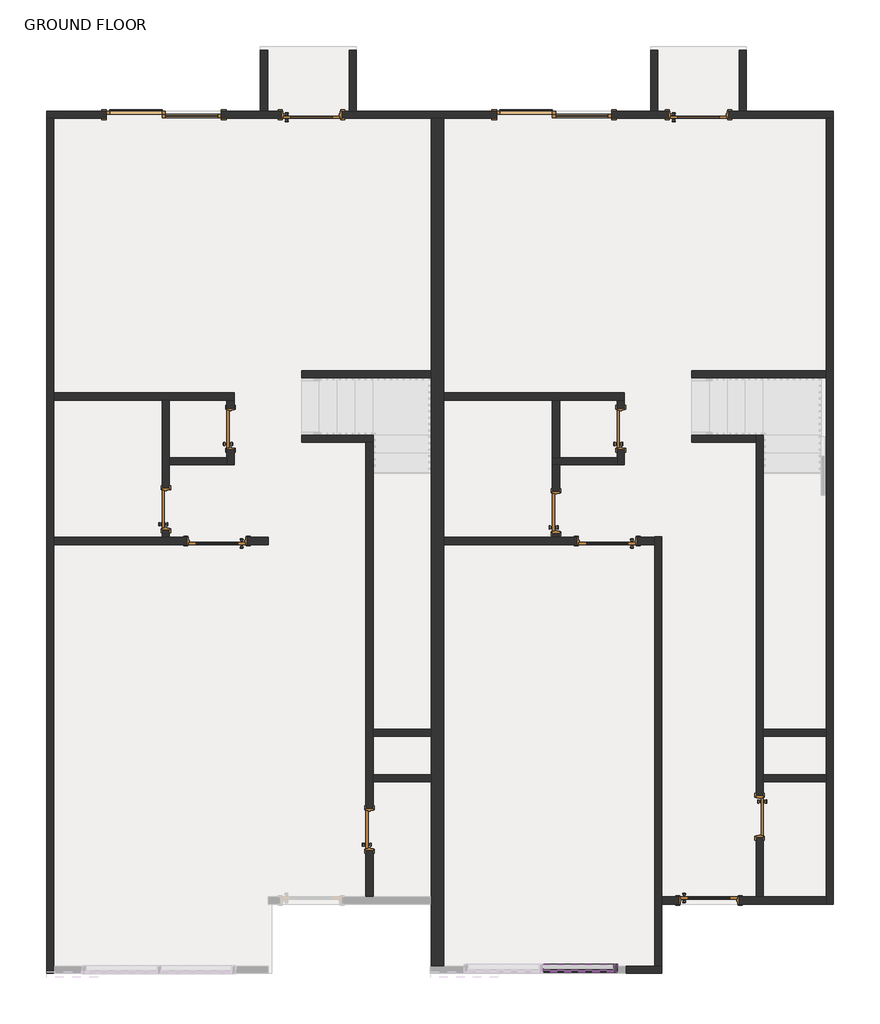
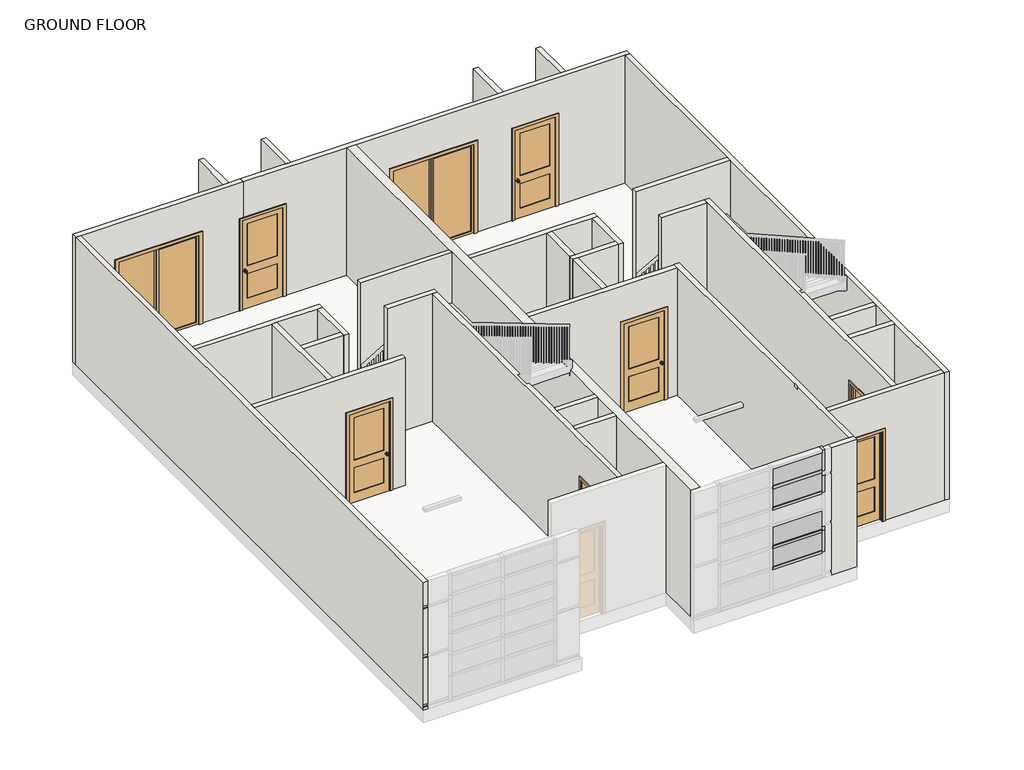
# One storey, part 2 of 4: 33 walls, 13 doors, 8 members, 4 plates.
"""IFC4 building model written with IfcOpenShell, lengths in millimetres."""

from ifc_helpers import new_model, si_unit, frame, origin, place, context, project, spatial, polyline, outline, extrude, faceted_brep, transform, mapped, element, save
from components import door_166d4031, door_049a69ed, door_d4071c8b, door_c25f678d, member_866a01fa, member_7cfea1b5, member_7fd687a9, member_fb13da3b, system_panel_glazed_162183a4, system_panel_glazed_09ecb9ef, system_panel_glazed_28d744da, system_panel_glazed_d671f7fc

model = new_model("IFC4")

# Units and contexts
model_context = context("Model", 3, world=origin())
ifc_project = project(units=[si_unit("LENGTHUNIT", "METRE", prefix="MILLI")], contexts=[model_context])

# Site, building, storey
site = spatial("IfcSite", under=ifc_project)
building = spatial("IfcBuilding", under=site)
storey = spatial("IfcBuildingStorey", under=building, Name="GROUND FLOOR", Elevation=304.8)

# Doors
placement = place(None, origin())
door_shape = door_166d4031(model_context)
element("IfcDoor", 1, ObjectType="Door-Double-Sliding : 72\" x 84\"", at=placement, inside=storey, context=model_context, shape_type="MappedRepresentation", body=[
    mapped(door_shape, transform((-16396.3007021, 8102.2409199, 304.8), x_axis=(1.0, 0.0, 0.0), y_axis=(0.0, 1.0, 0.0), z_axis=(0.0, 0.0, 1.0))),
])
element("IfcDoor", 2, ObjectType="Door-Double-Sliding : 72\" x 84\"", at=placement, inside=storey, context=model_context, shape_type="MappedRepresentation", body=[
    mapped(door_shape, transform((-10187.8860997, 8102.2409199, 304.8), x_axis=(1.0, 0.0, 0.0), y_axis=(0.0, 1.0, 0.0), z_axis=(0.0, 0.0, 1.0))),
])
door_2_shape = door_049a69ed(model_context)
element("IfcDoor", 3, ObjectType="Door-Interior-Single-2_Panel-Wood : 36\" x 84\"", at=placement, inside=storey, context=model_context, shape_type="MappedRepresentation", body=[
    mapped(door_2_shape, transform((-14046.8007021, 8226.0659199, 304.8), x_axis=(1.0, 0.0, 0.0), y_axis=(0.0, 1.0, 0.0), z_axis=(0.0, 0.0, 1.0))),
])
element("IfcDoor", 4, ObjectType="Door-Interior-Single-2_Panel-Wood : 36\" x 84\"", at=placement, inside=storey, context=model_context, shape_type="MappedRepresentation", body=[
    mapped(door_2_shape, transform((-7889.1860997, 8226.0659199, 304.8), x_axis=(1.0, 0.0, 0.0), y_axis=(0.0, 1.0, 0.0), z_axis=(0.0, 0.0, 1.0))),
])
door_3_shape = door_d4071c8b(model_context)
element("IfcDoor", 5, ObjectType="Door-Interior-Single-2_Panel-Wood : 36\" x 84\"", at=placement, inside=storey, context=model_context, shape_type="MappedRepresentation", body=[
    mapped(door_3_shape, transform((-15551.7507021, 1444.2659199, 304.8), x_axis=(-1.0, 0.0, 0.0), y_axis=(0.0, -1.0, 0.0), z_axis=(0.0, 0.0, 1.0))),
])
element("IfcDoor", 6, ObjectType="Door-Interior-Single-2_Panel-Wood : 36\" x 84\"", at=placement, inside=storey, context=model_context, shape_type="MappedRepresentation", body=[
    mapped(door_3_shape, transform((-9343.3360997, 1444.2659199, 304.8), x_axis=(-1.0, 0.0, 0.0), y_axis=(0.0, -1.0, 0.0), z_axis=(0.0, 0.0, 1.0))),
])
element("IfcDoor", 7, ObjectType="Door-Interior-Single-2_Panel-Wood : 36\" x 84\"", at=placement, inside=storey, context=model_context, shape_type="MappedRepresentation", body=[
    mapped(door_3_shape, transform((-7724.0860997, -4269.4090831, 304.8), x_axis=(1.0, 0.0, 0.0), y_axis=(0.0, 1.0, 0.0), z_axis=(0.0, 0.0, 1.0))),
])
door_4_shape = door_c25f678d(model_context)
element("IfcDoor", 8, ObjectType="Door-Interior-Single-Flush_Panel-Wood : 24\" x 84\"", at=placement, inside=storey, context=model_context, shape_type="MappedRepresentation", body=[
    mapped(door_4_shape, transform((-16367.7257021, 1955.4409199, 304.8), x_axis=(0.0, 1.0, 0.0), y_axis=(-1.0, 0.0, 0.0), z_axis=(0.0, 0.0, 1.0))),
])
element("IfcDoor", 9, ObjectType="Door-Interior-Single-Flush_Panel-Wood : 24\" x 84\"", at=placement, inside=storey, context=model_context, shape_type="MappedRepresentation", body=[
    mapped(door_4_shape, transform((-15339.0257021, 3231.7909199, 304.8), x_axis=(0.0, 1.0, 0.0), y_axis=(-1.0, 0.0, 0.0), z_axis=(0.0, 0.0, 1.0))),
])
element("IfcDoor", 10, ObjectType="Door-Interior-Single-Flush_Panel-Wood : 24\" x 84\"", at=placement, inside=storey, context=model_context, shape_type="MappedRepresentation", body=[
    mapped(door_4_shape, transform((-10159.3110997, 1904.6409199, 304.8), x_axis=(0.0, 1.0, 0.0), y_axis=(-1.0, 0.0, 0.0), z_axis=(0.0, 0.0, 1.0))),
])
element("IfcDoor", 11, ObjectType="Door-Interior-Single-Flush_Panel-Wood : 24\" x 84\"", at=placement, inside=storey, context=model_context, shape_type="MappedRepresentation", body=[
    mapped(door_4_shape, transform((-9130.6110998, 3231.7909199, 304.8), x_axis=(0.0, 1.0, 0.0), y_axis=(-1.0, 0.0, 0.0), z_axis=(0.0, 0.0, 1.0))),
])
element("IfcDoor", 12, ObjectType="Door-Interior-Single-Flush_Panel-Wood : 24\" x 84\"", at=placement, inside=storey, context=model_context, shape_type="MappedRepresentation", body=[
    mapped(door_4_shape, transform((-13129.2257021, -3142.284083, 304.8), x_axis=(0.0, 1.0, 0.0), y_axis=(-1.0, 0.0, 0.0), z_axis=(0.0, 0.0, 1.0))),
])
element("IfcDoor", 13, ObjectType="Door-Interior-Single-Flush_Panel-Wood : 24\" x 84\"", at=placement, inside=storey, context=model_context, shape_type="MappedRepresentation", body=[
    mapped(door_4_shape, transform((-6914.4610997, -2939.0840831, 304.8), x_axis=(0.0, -1.0, 0.0), y_axis=(1.0, 0.0, 0.0), z_axis=(0.0, 0.0, 1.0))),
])

# Members
member_shape = member_866a01fa(model_context)
element("IfcMember", 14, ObjectType="Rectangular Mullion : 2.5\" x 5\" rectangular", at=placement, inside=storey, context=model_context, shape_type="MappedRepresentation", body=[
    mapped(member_shape, transform((-9240.0344894, -5353.4090801, 2336.8), x_axis=(0.0, 0.0, 1.0), y_axis=(0.0, -1.0, 0.0), z_axis=(1.0, 0.0, 0.0))),
])
element("IfcMember", 15, ObjectType="Rectangular Mullion : 2.5\" x 5\" rectangular", at=placement, inside=storey, context=model_context, shape_type="MappedRepresentation", body=[
    mapped(member_shape, transform((-9240.0344894, -5353.4090801, 914.4), x_axis=(0.0, 0.0, 1.0), y_axis=(0.0, -1.0, 0.0), z_axis=(1.0, 0.0, 0.0))),
])
element("IfcMember", 16, ObjectType="Rectangular Mullion : 2.5\" x 5\" rectangular", at=placement, inside=storey, context=model_context, shape_type="MappedRepresentation", body=[
    mapped(member_shape, transform((-9240.0344894, -5353.4090801, 2844.8), x_axis=(0.0, 0.0, 1.0), y_axis=(0.0, -1.0, 0.0), z_axis=(1.0, 0.0, 0.0))),
])
element("IfcMember", 17, ObjectType="Rectangular Mullion : 2.5\" x 5\" rectangular", at=placement, inside=storey, context=model_context, shape_type="MappedRepresentation", body=[
    mapped(member_shape, transform((-9240.0344894, -5353.4090801, 1422.4), x_axis=(0.0, 0.0, 1.0), y_axis=(0.0, -1.0, 0.0), z_axis=(1.0, 0.0, 0.0))),
])
member_2_shape = member_7cfea1b5(model_context)
element("IfcMember", 18, ObjectType="Rectangular Mullion : 2.5\" x 5\" rectangular", at=placement, inside=storey, context=model_context, shape_type="MappedRepresentation", body=[
    mapped(member_2_shape, transform((-9176.5344894, -5353.4090801, 2336.8), x_axis=(1.0, 0.0, 0.0), y_axis=(0.0, -1.0, 0.0), z_axis=(0.0, 0.0, -1.0))),
])
member_3_shape = member_7fd687a9(model_context)
element("IfcMember", 19, ObjectType="Rectangular Mullion : 2.5\" x 5\" rectangular", at=placement, inside=storey, context=model_context, shape_type="MappedRepresentation", body=[
    mapped(member_3_shape, transform((-9176.5344894, -5353.4090801, 2844.8), x_axis=(1.0, 0.0, 0.0), y_axis=(0.0, -1.0, 0.0), z_axis=(0.0, 0.0, -1.0))),
])
element("IfcMember", 20, ObjectType="Rectangular Mullion : 2.5\" x 5\" rectangular", at=placement, inside=storey, context=model_context, shape_type="MappedRepresentation", body=[
    mapped(member_3_shape, transform((-9176.5344894, -5353.4090801, 914.4), x_axis=(1.0, 0.0, 0.0), y_axis=(0.0, -1.0, 0.0), z_axis=(0.0, 0.0, -1.0))),
])
member_4_shape = member_fb13da3b(model_context)
element("IfcMember", 21, ObjectType="Rectangular Mullion : 2.5\" x 5\" rectangular", at=placement, inside=storey, context=model_context, shape_type="MappedRepresentation", body=[
    mapped(member_4_shape, transform((-9176.5344894, -5353.4090801, 1422.4), x_axis=(1.0, 0.0, 0.0), y_axis=(0.0, -1.0, 0.0), z_axis=(0.0, 0.0, -1.0))),
])

# Plates
system_panel_glazed_shape = system_panel_glazed_162183a4(model_context)
element("IfcPlate", 22, ObjectType="System Panel : Glazed", at=placement, inside=storey, context=model_context, shape_type="MappedRepresentation", body=[
    mapped(system_panel_glazed_shape, transform((-9802.0094894, -5353.4090801, 2368.55), x_axis=(1.0, 0.0, 0.0), y_axis=(0.0, 1.0, 0.0), z_axis=(0.0, 0.0, 1.0))),
])
system_panel_glazed_2_shape = system_panel_glazed_09ecb9ef(model_context)
element("IfcPlate", 23, ObjectType="System Panel : Glazed", at=placement, inside=storey, context=model_context, shape_type="MappedRepresentation", body=[
    mapped(system_panel_glazed_2_shape, transform((-9802.0094894, -5353.4090801, 2876.55), x_axis=(1.0, 0.0, 0.0), y_axis=(0.0, 1.0, 0.0), z_axis=(0.0, 0.0, 1.0))),
])
system_panel_glazed_3_shape = system_panel_glazed_28d744da(model_context)
element("IfcPlate", 24, ObjectType="System Panel : Glazed", at=placement, inside=storey, context=model_context, shape_type="MappedRepresentation", body=[
    mapped(system_panel_glazed_3_shape, transform((-9802.0094894, -5353.4090801, 946.15), x_axis=(1.0, 0.0, 0.0), y_axis=(0.0, 1.0, 0.0), z_axis=(0.0, 0.0, 1.0))),
])
system_panel_glazed_4_shape = system_panel_glazed_d671f7fc(model_context)
element("IfcPlate", 25, ObjectType="System Panel : Glazed", at=placement, inside=storey, context=model_context, shape_type="MappedRepresentation", body=[
    mapped(system_panel_glazed_4_shape, transform((-9802.0094894, -5353.4090801, 1454.15), x_axis=(1.0, 0.0, 0.0), y_axis=(0.0, 1.0, 0.0), z_axis=(0.0, 0.0, 1.0))),
])

# Walls
element("IfcWall", 26, at=placement, inside=storey, context=model_context, shape_type="Brep", body=[
    faceted_brep([(-18263.2007021, 8286.3909199, 3352.8), (-14859.6007021, 8286.3909199, 3352.8), (-14745.3007021, 8286.3909199, 3352.8), (-14478.6007021, 8286.3909199, 3352.8), (-14478.6007021, 8286.3909199, 2463.8), (-14529.4007021, 8286.3909199, 2463.8), (-14529.4007021, 8286.3909199, 304.8), (-14745.3007021, 8286.3909199, 304.8), (-14859.6007021, 8286.3909199, 304.8), (-15481.9007021, 8286.3909199, 304.8), (-15481.9007021, 8286.3909199, 2438.4), (-17310.7007021, 8286.3909199, 2438.4), (-17310.7007021, 8286.3909199, 304.8), (-18263.2007021, 8286.3909199, 304.8), (-14478.6007021, 8172.0909199, 3352.8), (-18148.9007021, 8172.0909199, 3352.8), (-18263.2007021, 8172.0909199, 3352.8), (-18263.2007021, 8172.0909199, 304.8), (-18148.9007021, 8172.0909199, 304.8), (-17310.7007021, 8172.0909199, 304.8), (-17310.7007021, 8172.0909199, 2438.4), (-15481.9007021, 8172.0909199, 2438.4), (-15481.9007021, 8172.0909199, 304.8), (-14529.4007021, 8172.0909199, 304.8), (-14529.4007021, 8172.0909199, 2463.8), (-14478.6007021, 8172.0909199, 2463.8)], [[[0, 1, 2, 3, 4, 5, 6, 7, 8, 9, 10, 11, 12, 13]], [[14, 15, 16, 17, 18, 19, 20, 21, 22, 23, 24, 25]], [[17, 13, 12, 19, 18]], [[22, 9, 8, 7, 6, 23]], [[3, 2, 1, 0, 16, 15, 14]], [[3, 14, 25, 4]], [[0, 13, 17, 16]], [[12, 11, 20, 19]], [[10, 9, 22, 21]], [[11, 10, 21, 20]], [[24, 5, 4, 25]], [[5, 24, 23, 6]]]),
])
element("IfcWall", 27, at=placement, inside=storey, context=model_context, shape_type="Brep", body=[
    faceted_brep([(-18263.2007021, 8172.0909199, 304.8), (-18263.2007021, -5429.6090801, 304.8), (-18263.2007021, -5429.6090801, 368.3), (-18263.2007021, -5404.2090801, 368.3), (-18263.2007021, -5404.2090801, 436.0333333), (-18263.2007021, -5429.6090801, 436.0333333), (-18263.2007021, -5429.6090801, 1544.32), (-18263.2007021, -5404.2090801, 1544.32), (-18263.2007021, -5404.2090801, 1612.0533333), (-18263.2007021, -5429.6090801, 1612.0533333), (-18263.2007021, -5429.6090801, 2720.34), (-18263.2007021, -5404.2090801, 2720.34), (-18263.2007021, -5404.2090801, 2788.0733333), (-18263.2007021, -5429.6090801, 2788.0733333), (-18263.2007021, -5429.6090801, 3352.8), (-18263.2007021, 8172.0909199, 3352.8), (-18148.9007021, -5429.6090801, 304.8), (-18148.9007021, -5315.3090801, 304.8), (-18148.9007021, 1390.2909199, 304.8), (-18148.9007021, 1504.5909199, 304.8), (-18148.9007021, 3688.9909199, 304.8), (-18148.9007021, 3803.2909199, 304.8), (-18148.9007021, 8172.0909199, 304.8), (-18148.9007021, 8172.0909199, 3352.8), (-18148.9007021, 3803.2909199, 3352.8), (-18148.9007021, 3688.9909199, 3352.8), (-18148.9007021, 1504.5909199, 3352.8), (-18148.9007021, 1390.2909199, 3352.8), (-18148.9007021, -5315.3090801, 3352.8), (-18148.9007021, -5429.6090801, 3352.8), (-18148.9007021, -5429.6090801, 2788.0733333), (-18148.9007021, -5404.2090801, 2788.0733333), (-18148.9007021, -5404.2090801, 2720.34), (-18148.9007021, -5429.6090801, 2720.34), (-18148.9007021, -5429.6090801, 1612.0533333), (-18148.9007021, -5404.2090801, 1612.0533333), (-18148.9007021, -5404.2090801, 1544.32), (-18148.9007021, -5429.6090801, 1544.32), (-18148.9007021, -5429.6090801, 436.0333333), (-18148.9007021, -5404.2090801, 436.0333333), (-18148.9007021, -5404.2090801, 368.3), (-18148.9007021, -5429.6090801, 368.3)], [[[0, 1, 2, 3, 4, 5, 6, 7, 8, 9, 10, 11, 12, 13, 14, 15]], [[16, 17, 18, 19, 20, 21, 22, 23, 24, 25, 26, 27, 28, 29, 30, 31, 32, 33, 34, 35, 36, 37, 38, 39, 40, 41]], [[1, 0, 22, 21, 20, 19, 18, 17, 16]], [[15, 14, 29, 28, 27, 26, 25, 24, 23]], [[0, 15, 23, 22]], [[1, 16, 41, 2]], [[29, 14, 13, 30]], [[5, 38, 37, 6]], [[9, 34, 33, 10]], [[39, 4, 3, 40]], [[40, 3, 2, 41]], [[4, 39, 38, 5]], [[35, 8, 7, 36]], [[36, 7, 6, 37]], [[8, 35, 34, 9]], [[31, 12, 11, 32]], [[32, 11, 10, 33]], [[12, 31, 30, 13]]]),
])
element("IfcWall", 28, at=placement, inside=storey, context=model_context, shape_type="Brep", body=[
    faceted_brep([(-14738.9507021, 1390.2909199, 304.8), (-14738.9507021, 1390.2909199, 3352.8), (-18148.9007021, 1390.2909199, 3352.8), (-18148.9007021, 1390.2909199, 304.8), (-16034.3507021, 1390.2909199, 304.8), (-16034.3507021, 1390.2909199, 2463.8), (-15069.1507021, 1390.2909199, 2463.8), (-15069.1507021, 1390.2909199, 304.8), (-14738.9507021, 1504.5909199, 3352.8), (-14738.9507021, 1504.5909199, 304.8), (-15069.1507021, 1504.5909199, 304.8), (-15069.1507021, 1504.5909199, 2463.8), (-16034.3507021, 1504.5909199, 2463.8), (-16034.3507021, 1504.5909199, 304.8), (-16307.4007021, 1504.5909199, 304.8), (-16421.7007021, 1504.5909199, 304.8), (-18148.9007021, 1504.5909199, 304.8), (-18148.9007021, 1504.5909199, 3352.8), (-16421.7007021, 1504.5909199, 3352.8), (-16307.4007021, 1504.5909199, 3352.8)], [[[0, 1, 2, 3, 4, 5, 6, 7]], [[8, 9, 10, 11, 12, 13, 14, 15, 16, 17, 18, 19]], [[9, 0, 7, 10]], [[3, 16, 15, 14, 13, 4]], [[1, 0, 9, 8]], [[2, 1, 8, 19, 18, 17]], [[3, 2, 17, 16]], [[12, 5, 4, 13]], [[5, 12, 11, 6]], [[6, 11, 10, 7]]]),
])
element("IfcWall", 29, at=placement, inside=storey, context=model_context, shape_type="Brep", body=[
    faceted_brep([(-18148.9007021, 3688.9909199, 304.8), (-16421.7007021, 3688.9909199, 304.8), (-16307.4007021, 3688.9909199, 304.8), (-15393.0007021, 3688.9909199, 304.8), (-15278.7007021, 3688.9909199, 304.8), (-15278.7007021, 3688.9909199, 3352.8), (-15393.0007021, 3688.9909199, 3352.8), (-16307.4007021, 3688.9909199, 3352.8), (-16421.7007021, 3688.9909199, 3352.8), (-18148.9007021, 3688.9909199, 3352.8), (-18148.9007021, 3803.2909199, 304.8), (-18148.9007021, 3803.2909199, 3352.8), (-15278.7007021, 3803.2909199, 3352.8), (-15278.7007021, 3803.2909199, 304.8)], [[[0, 1, 2, 3, 4, 5, 6, 7, 8, 9]], [[10, 11, 12, 13]], [[4, 3, 2, 1, 0, 10, 13]], [[9, 8, 7, 6, 5, 12, 11]], [[0, 9, 11, 10]], [[5, 4, 13, 12]]]),
])
element("IfcWall", 30, at=placement, inside=storey, context=model_context, shape_type="Brep", body=[
    faceted_brep([(-15393.0007021, 2660.2909199, 3352.8), (-15393.0007021, 2774.5909199, 3352.8), (-15393.0007021, 3688.9909199, 3352.8), (-15393.0007021, 3688.9909199, 304.8), (-15393.0007021, 3561.9909199, 304.8), (-15393.0007021, 3561.9909199, 2463.8), (-15393.0007021, 2901.5909199, 2463.8), (-15393.0007021, 2901.5909199, 304.8), (-15393.0007021, 2774.5909199, 304.8), (-15393.0007021, 2660.2909199, 304.8), (-15278.7007021, 3688.9909199, 3352.8), (-15278.7007021, 2660.2909199, 3352.8), (-15278.7007021, 2660.2909199, 304.8), (-15278.7007021, 2901.5909199, 304.8), (-15278.7007021, 2901.5909199, 2463.8), (-15278.7007021, 3561.9909199, 2463.8), (-15278.7007021, 3561.9909199, 304.8), (-15278.7007021, 3688.9909199, 304.8)], [[[0, 1, 2, 3, 4, 5, 6, 7, 8, 9]], [[10, 11, 12, 13, 14, 15, 16, 17]], [[3, 17, 16, 4]], [[12, 9, 8, 7, 13]], [[2, 1, 0, 11, 10]], [[3, 2, 10, 17]], [[0, 9, 12, 11]], [[15, 5, 4, 16]], [[5, 15, 14, 6]], [[6, 14, 13, 7]]]),
])
element("IfcWall", 31, at=placement, inside=storey, context=model_context, shape_type="SweptSolid", body=[
    extrude(outline(polyline([(-16307.4007021, 2774.5909199), (-15393.0007021, 2774.5909199), (-15393.0007021, 2660.2909199), (-16307.4007021, 2660.2909199), (-16307.4007021, 2774.5909199)])), frame((0.0, 0.0, 304.8), z_axis=(0.0, 0.0, 1.0), x_axis=(1.0, 0.0, 0.0)), (0.0, 0.0, 1.0), 3048.0),
])
element("IfcWall", 32, at=placement, inside=storey, context=model_context, shape_type="Brep", body=[
    faceted_brep([(-16421.7007021, 1504.5909199, 3352.8), (-16421.7007021, 3688.9909199, 3352.8), (-16421.7007021, 3688.9909199, 304.8), (-16421.7007021, 2285.6409199, 304.8), (-16421.7007021, 2285.6409199, 2463.8), (-16421.7007021, 1625.2409199, 2463.8), (-16421.7007021, 1625.2409199, 304.8), (-16421.7007021, 1504.5909199, 304.8), (-16307.4007021, 3688.9909199, 3352.8), (-16307.4007021, 2774.5909199, 3352.8), (-16307.4007021, 2660.2909199, 3352.8), (-16307.4007021, 1504.5909199, 3352.8), (-16307.4007021, 1504.5909199, 304.8), (-16307.4007021, 1625.2409199, 304.8), (-16307.4007021, 1625.2409199, 2463.8), (-16307.4007021, 2285.6409199, 2463.8), (-16307.4007021, 2285.6409199, 304.8), (-16307.4007021, 2660.2909199, 304.8), (-16307.4007021, 2774.5909199, 304.8), (-16307.4007021, 3688.9909199, 304.8)], [[[0, 1, 2, 3, 4, 5, 6, 7]], [[8, 9, 10, 11, 12, 13, 14, 15, 16, 17, 18, 19]], [[2, 19, 18, 17, 16, 3]], [[12, 7, 6, 13]], [[1, 0, 11, 10, 9, 8]], [[0, 7, 12, 11]], [[2, 1, 8, 19]], [[15, 4, 3, 16]], [[4, 15, 14, 5]], [[5, 14, 13, 6]]]),
])
element("IfcWall", 33, at=placement, inside=storey, context=model_context, shape_type="Brep", body=[
    faceted_brep([(-5742.8860997, 8172.0909199, 3352.8), (-5857.1860997, 8172.0909199, 3352.8), (-11940.4860997, 8172.0909199, 3352.8), (-12143.6860997, 8172.0909199, 3352.8), (-14478.6007021, 8172.0909199, 3352.8), (-14478.6007021, 8172.0909199, 2463.8), (-13564.2007021, 8172.0909199, 2463.8), (-13564.2007021, 8172.0909199, 304.8), (-12143.6860997, 8172.0909199, 304.8), (-11940.4860997, 8172.0909199, 304.8), (-11102.2860997, 8172.0909199, 304.8), (-11102.2860997, 8172.0909199, 2438.4), (-9273.4860997, 8172.0909199, 2438.4), (-9273.4860997, 8172.0909199, 304.8), (-8371.7860997, 8172.0909199, 304.8), (-8371.7860997, 8172.0909199, 2463.8), (-7406.5860997, 8172.0909199, 2463.8), (-7406.5860997, 8172.0909199, 304.8), (-5857.1860997, 8172.0909199, 304.8), (-5742.8860997, 8172.0909199, 304.8), (-14478.6007021, 8286.3909199, 3352.8), (-13449.9007021, 8286.3909199, 3352.8), (-13335.6007021, 8286.3909199, 3352.8), (-8651.1860997, 8286.3909199, 3352.8), (-8536.8860997, 8286.3909199, 3352.8), (-7241.4860997, 8286.3909199, 3352.8), (-7127.1860997, 8286.3909199, 3352.8), (-5742.8860997, 8286.3909199, 3352.8), (-5742.8860997, 8286.3909199, 304.8), (-7127.1860997, 8286.3909199, 304.8), (-7241.4860997, 8286.3909199, 304.8), (-7406.5860997, 8286.3909199, 304.8), (-7406.5860997, 8286.3909199, 2463.8), (-8371.7860997, 8286.3909199, 2463.8), (-8371.7860997, 8286.3909199, 304.8), (-8536.8860997, 8286.3909199, 304.8), (-8651.1860997, 8286.3909199, 304.8), (-9273.4860997, 8286.3909199, 304.8), (-9273.4860997, 8286.3909199, 2438.4), (-11102.2860997, 8286.3909199, 2438.4), (-11102.2860997, 8286.3909199, 304.8), (-13335.6007021, 8286.3909199, 304.8), (-13449.9007021, 8286.3909199, 304.8), (-13564.2007021, 8286.3909199, 304.8), (-13564.2007021, 8286.3909199, 2463.8), (-14478.6007021, 8286.3909199, 2463.8)], [[[0, 1, 2, 3, 4, 5, 6, 7, 8, 9, 10, 11, 12, 13, 14, 15, 16, 17, 18, 19]], [[20, 21, 22, 23, 24, 25, 26, 27, 28, 29, 30, 31, 32, 33, 34, 35, 36, 37, 38, 39, 40, 41, 42, 43, 44, 45]], [[28, 19, 18, 17, 31, 30, 29]], [[40, 10, 9, 8, 7, 43, 42, 41]], [[13, 37, 36, 35, 34, 14]], [[4, 3, 2, 1, 0, 27, 26, 25, 24, 23, 22, 21, 20]], [[4, 20, 45, 5]], [[0, 19, 28, 27]], [[40, 39, 11, 10]], [[38, 37, 13, 12]], [[39, 38, 12, 11]], [[6, 44, 43, 7]], [[44, 6, 5, 45]], [[16, 32, 31, 17]], [[32, 16, 15, 33]], [[33, 15, 14, 34]]]),
])
element("IfcWall", 34, at=placement, inside=storey, context=model_context, shape_type="Brep", body=[
    faceted_brep([(-5857.1860997, 8172.0909199, 304.8), (-5857.1860997, 4158.8909199, 304.8), (-5857.1860997, 4044.5909199, 304.8), (-5857.1860997, -1548.4340831, 304.8), (-5857.1860997, -1662.7340831, 304.8), (-5857.1860997, -2272.3340831, 304.8), (-5857.1860997, -2386.6340831, 304.8), (-5857.1860997, -4215.4340831, 304.8), (-5857.1860997, -4329.7340831, 304.8), (-5857.1860997, -4329.7340831, 3352.8), (-5857.1860997, -4215.4340831, 3352.8), (-5857.1860997, -2386.6340831, 3352.8), (-5857.1860997, -2272.3340831, 3352.8), (-5857.1860997, -1662.7340831, 3352.8), (-5857.1860997, -1548.4340831, 3352.8), (-5857.1860997, 4044.5909199, 3352.8), (-5857.1860997, 4158.8909199, 3352.8), (-5857.1860997, 8172.0909199, 3352.8), (-5742.8860997, 8172.0909199, 304.8), (-5742.8860997, 8172.0909199, 3352.8), (-5742.8860997, -4329.7340831, 3352.8), (-5742.8860997, -4329.7340831, 304.8)], [[[0, 1, 2, 3, 4, 5, 6, 7, 8, 9, 10, 11, 12, 13, 14, 15, 16, 17]], [[18, 19, 20, 21]], [[8, 7, 6, 5, 4, 3, 2, 1, 0, 18, 21]], [[17, 16, 15, 14, 13, 12, 11, 10, 9, 20, 19]], [[0, 17, 19, 18]], [[9, 8, 21, 20]]]),
])
element("IfcWall", 35, at=placement, inside=storey, context=model_context, shape_type="Brep", body=[
    faceted_brep([(-8473.3860997, -4215.4340831, 3352.8), (-6974.7860997, -4215.4340831, 3352.8), (-6860.4860997, -4215.4340831, 3352.8), (-5857.1860997, -4215.4340831, 3352.8), (-5857.1860997, -4215.4340831, 304.8), (-6860.4860997, -4215.4340831, 304.8), (-6974.7860997, -4215.4340831, 304.8), (-7241.4860997, -4215.4340831, 304.8), (-7241.4860997, -4215.4340831, 2463.8), (-8206.6860997, -4215.4340831, 2463.8), (-8206.6860997, -4215.4340831, 304.8), (-8473.3860997, -4215.4340831, 304.8), (-5857.1860997, -4329.7340831, 3352.8), (-8473.3860997, -4329.7340831, 3352.8), (-8473.3860997, -4329.7340831, 304.8), (-8206.6860997, -4329.7340831, 304.8), (-8206.6860997, -4329.7340831, 2463.8), (-7241.4860997, -4329.7340831, 2463.8), (-7241.4860997, -4329.7340831, 304.8), (-5857.1860997, -4329.7340831, 304.8)], [[[0, 1, 2, 3, 4, 5, 6, 7, 8, 9, 10, 11]], [[12, 13, 14, 15, 16, 17, 18, 19]], [[4, 19, 18, 7, 6, 5]], [[14, 11, 10, 15]], [[3, 2, 1, 0, 13, 12]], [[4, 3, 12, 19]], [[0, 11, 14, 13]], [[17, 8, 7, 18]], [[8, 17, 16, 9]], [[9, 16, 15, 10]]]),
])
element("IfcWall", 36, at=placement, inside=storey, context=model_context, shape_type="Brep", body=[
    faceted_brep([(-9044.8860997, -5429.6090801, 304.8), (-8473.3860997, -5429.6090801, 304.8), (-8473.3860997, -5429.6090801, 3352.8), (-9044.8860997, -5429.6090801, 3352.8), (-9044.8860997, -5429.6090801, 2788.0733333), (-9044.8860997, -5429.6090801, 2720.34), (-9044.8860997, -5429.6090801, 1612.0533333), (-9044.8860997, -5429.6090801, 1544.32), (-9044.8860997, -5429.6090801, 436.0333333), (-9044.8860997, -5429.6090801, 368.3), (-9044.8860997, -5315.3090801, 304.8), (-9044.8860997, -5315.3090801, 3352.8), (-8587.6860997, -5315.3090801, 3352.8), (-8473.3860997, -5315.3090801, 3352.8), (-8473.3860997, -5315.3090801, 304.8), (-8587.6860997, -5315.3090801, 304.8)], [[[0, 1, 2, 3, 4, 5, 6, 7, 8, 9]], [[10, 11, 12, 13, 14, 15]], [[1, 0, 10, 15, 14]], [[3, 2, 13, 12, 11]], [[0, 9, 8, 7, 6, 5, 4, 3, 11, 10]], [[2, 1, 14, 13]]]),
])
element("IfcWall", 37, at=placement, inside=storey, context=model_context, shape_type="Brep", body=[
    faceted_brep([(-8473.3860997, -5315.3090801, 304.8), (-8473.3860997, -4329.7340831, 304.8), (-8473.3860997, -4215.4340831, 304.8), (-8473.3860997, 1517.2909199, 304.8), (-8473.3860997, 1517.2909199, 3352.8), (-8473.3860997, -4215.4340831, 3352.8), (-8473.3860997, -4329.7340831, 3352.8), (-8473.3860997, -5315.3090801, 3352.8), (-8587.6860997, -5315.3090801, 304.8), (-8587.6860997, -5315.3090801, 3352.8), (-8587.6860997, 1390.2909199, 3352.8), (-8587.6860997, 1504.5909199, 3352.8), (-8587.6860997, 1517.2909199, 3352.8), (-8587.6860997, 1517.2909199, 304.8), (-8587.6860997, 1504.5909199, 304.8), (-8587.6860997, 1390.2909199, 304.8)], [[[0, 1, 2, 3, 4, 5, 6, 7]], [[8, 9, 10, 11, 12, 13, 14, 15]], [[3, 2, 1, 0, 8, 15, 14, 13]], [[4, 3, 13, 12]], [[7, 6, 5, 4, 12, 11, 10, 9]], [[0, 7, 9, 8]]]),
])
element("IfcWall", 38, at=placement, inside=storey, context=model_context, shape_type="Brep", body=[
    faceted_brep([(-8587.6860997, 1390.2909199, 3352.8), (-11940.4860997, 1390.2909199, 3352.8), (-11940.4860997, 1390.2909199, 304.8), (-9825.9360997, 1390.2909199, 304.8), (-9825.9360997, 1390.2909199, 2463.8), (-8860.7360997, 1390.2909199, 2463.8), (-8860.7360997, 1390.2909199, 304.8), (-8587.6860997, 1390.2909199, 304.8), (-11940.4860997, 1504.5909199, 3352.8), (-10213.2860997, 1504.5909199, 3352.8), (-10098.9860997, 1504.5909199, 3352.8), (-8587.6860997, 1504.5909199, 3352.8), (-8587.6860997, 1504.5909199, 304.8), (-8860.7360997, 1504.5909199, 304.8), (-8860.7360997, 1504.5909199, 2463.8), (-9825.9360997, 1504.5909199, 2463.8), (-9825.9360997, 1504.5909199, 304.8), (-10098.9860997, 1504.5909199, 304.8), (-10213.2860997, 1504.5909199, 304.8), (-11940.4860997, 1504.5909199, 304.8)], [[[0, 1, 2, 3, 4, 5, 6, 7]], [[8, 9, 10, 11, 12, 13, 14, 15, 16, 17, 18, 19]], [[12, 7, 6, 13]], [[2, 19, 18, 17, 16, 3]], [[1, 0, 11, 10, 9, 8]], [[0, 7, 12, 11]], [[2, 1, 8, 19]], [[15, 4, 3, 16]], [[4, 15, 14, 5]], [[5, 14, 13, 6]]]),
])
element("IfcWall", 39, at=placement, inside=storey, context=model_context, shape_type="Brep", body=[
    faceted_brep([(-12143.6860997, 8172.0909199, 304.8), (-12143.6860997, 4158.8909199, 304.8), (-12143.6860997, 4044.5909199, 304.8), (-12143.6860997, -1548.4340831, 304.8), (-12143.6860997, -1662.7340831, 304.8), (-12143.6860997, -2272.334083, 304.8), (-12143.6860997, -2386.634083, 304.8), (-12143.6860997, -4215.434083, 304.8), (-12143.6860997, -4329.734083, 304.8), (-12143.6860997, -5315.3090801, 304.8), (-12143.6860997, -5315.3090801, 3352.8), (-12143.6860997, -4329.734083, 3352.8), (-12143.6860997, -4215.434083, 3352.8), (-12143.6860997, -2386.634083, 3352.8), (-12143.6860997, -2272.334083, 3352.8), (-12143.6860997, -1662.7340831, 3352.8), (-12143.6860997, -1548.4340831, 3352.8), (-12143.6860997, 4044.5909199, 3352.8), (-12143.6860997, 4158.8909199, 3352.8), (-12143.6860997, 8172.0909199, 3352.8), (-11940.4860997, 8172.0909199, 304.8), (-11940.4860997, 8172.0909199, 3352.8), (-11940.4860997, 3803.2909199, 3352.8), (-11940.4860997, 3688.9909199, 3352.8), (-11940.4860997, 1504.5909199, 3352.8), (-11940.4860997, 1390.2909199, 3352.8), (-11940.4860997, -5315.3090801, 3352.8), (-11940.4860997, -5315.3090801, 304.8), (-11940.4860997, 1390.2909199, 304.8), (-11940.4860997, 1504.5909199, 304.8), (-11940.4860997, 3688.9909199, 304.8), (-11940.4860997, 3803.2909199, 304.8)], [[[0, 1, 2, 3, 4, 5, 6, 7, 8, 9, 10, 11, 12, 13, 14, 15, 16, 17, 18, 19]], [[20, 21, 22, 23, 24, 25, 26, 27, 28, 29, 30, 31]], [[9, 8, 7, 6, 5, 4, 3, 2, 1, 0, 20, 31, 30, 29, 28, 27]], [[19, 18, 17, 16, 15, 14, 13, 12, 11, 10, 26, 25, 24, 23, 22, 21]], [[0, 19, 21, 20]], [[10, 9, 27, 26]]]),
])
element("IfcWall", 40, at=placement, inside=storey, context=model_context, shape_type="SweptSolid", body=[
    extrude(outline(polyline([(-14204.9595293, 4158.8909199), (-12143.6860997, 4158.8909199), (-12143.6860997, 4044.5909199), (-14204.9595293, 4044.5909199), (-14204.9595293, 4158.8909199)])), frame((0.0, 0.0, 304.8), z_axis=(0.0, 0.0, 1.0), x_axis=(1.0, 0.0, 0.0)), (0.0, 0.0, 1.0), 3048.0),
])
element("IfcWall", 41, at=placement, inside=storey, context=model_context, shape_type="Brep", body=[
    faceted_brep([(-14204.9595293, 3015.8909199, 304.8), (-13183.2007021, 3015.8909199, 304.8), (-13068.9007021, 3015.8909199, 304.8), (-13068.9007021, 3015.8909199, 3352.8), (-13183.2007021, 3015.8909199, 3352.8), (-14204.9595293, 3015.8909199, 3352.8), (-14204.9595293, 3130.1909199, 304.8), (-14204.9595293, 3130.1909199, 3352.8), (-13068.9007021, 3130.1909199, 3352.8), (-13068.9007021, 3130.1909199, 304.8)], [[[0, 1, 2, 3, 4, 5]], [[6, 7, 8, 9]], [[2, 1, 0, 6, 9]], [[5, 4, 3, 8, 7]], [[0, 5, 7, 6]], [[3, 2, 9, 8]]]),
])
element("IfcWall", 42, at=placement, inside=storey, context=model_context, shape_type="Brep", body=[
    faceted_brep([(-13183.2007021, -4215.434083, 3352.8), (-13183.2007021, 3015.8909199, 3352.8), (-13183.2007021, 3015.8909199, 304.8), (-13183.2007021, -2812.084083, 304.8), (-13183.2007021, -2812.084083, 2463.8), (-13183.2007021, -3472.484083, 2463.8), (-13183.2007021, -3472.484083, 304.8), (-13183.2007021, -4215.434083, 304.8), (-13068.9007021, 3015.8909199, 3352.8), (-13068.9007021, -1548.4340831, 3352.8), (-13068.9007021, -1662.7340831, 3352.8), (-13068.9007021, -2272.334083, 3352.8), (-13068.9007021, -2386.634083, 3352.8), (-13068.9007021, -4215.434083, 3352.8), (-13068.9007021, -4215.434083, 304.8), (-13068.9007021, -3472.484083, 304.8), (-13068.9007021, -3472.484083, 2463.8), (-13068.9007021, -2812.084083, 2463.8), (-13068.9007021, -2812.084083, 304.8), (-13068.9007021, -2386.634083, 304.8), (-13068.9007021, -2272.334083, 304.8), (-13068.9007021, -1662.7340831, 304.8), (-13068.9007021, -1548.4340831, 304.8), (-13068.9007021, 3015.8909199, 304.8)], [[[0, 1, 2, 3, 4, 5, 6, 7]], [[8, 9, 10, 11, 12, 13, 14, 15, 16, 17, 18, 19, 20, 21, 22, 23]], [[2, 23, 22, 21, 20, 19, 18, 3]], [[14, 7, 6, 15]], [[1, 0, 13, 12, 11, 10, 9, 8]], [[2, 1, 8, 23]], [[0, 7, 14, 13]], [[17, 4, 3, 18]], [[4, 17, 16, 5]], [[5, 16, 15, 6]]]),
])
element("IfcWall", 43, at=placement, inside=storey, context=model_context, shape_type="SweptSolid", body=[
    extrude(outline(polyline([(-12143.6860997, -1662.7340831), (-13068.9007021, -1662.7340831), (-13068.9007021, -1548.4340831), (-12143.6860997, -1548.4340831), (-12143.6860997, -1662.7340831)])), frame((0.0, 0.0, 304.8), z_axis=(0.0, 0.0, 1.0), x_axis=(1.0, 0.0, 0.0)), (0.0, 0.0, 1.0), 3048.0),
])
element("IfcWall", 44, at=placement, inside=storey, context=model_context, shape_type="SweptSolid", body=[
    extrude(outline(polyline([(-12143.6860997, -2386.634083), (-13068.9007021, -2386.634083), (-13068.9007021, -2272.334083), (-12143.6860997, -2272.334083), (-12143.6860997, -2386.634083)])), frame((0.0, 0.0, 304.8), z_axis=(0.0, 0.0, 1.0), x_axis=(1.0, 0.0, 0.0)), (0.0, 0.0, 1.0), 3048.0),
])
element("IfcWall", 45, at=placement, inside=storey, context=model_context, shape_type="Brep", body=[
    faceted_brep([(-11940.4860997, 3688.9909199, 304.8), (-10213.2860997, 3688.9909199, 304.8), (-10098.9860997, 3688.9909199, 304.8), (-9184.5860998, 3688.9909199, 304.8), (-9070.2860998, 3688.9909199, 304.8), (-9070.2860998, 3688.9909199, 3352.8), (-9184.5860998, 3688.9909199, 3352.8), (-10098.9860997, 3688.9909199, 3352.8), (-10213.2860997, 3688.9909199, 3352.8), (-11940.4860997, 3688.9909199, 3352.8), (-11940.4860997, 3803.2909199, 304.8), (-11940.4860997, 3803.2909199, 3352.8), (-9070.2860998, 3803.2909199, 3352.8), (-9070.2860998, 3803.2909199, 304.8)], [[[0, 1, 2, 3, 4, 5, 6, 7, 8, 9]], [[10, 11, 12, 13]], [[4, 3, 2, 1, 0, 10, 13]], [[9, 8, 7, 6, 5, 12, 11]], [[0, 9, 11, 10]], [[5, 4, 13, 12]]]),
])
element("IfcWall", 46, at=placement, inside=storey, context=model_context, shape_type="Brep", body=[
    faceted_brep([(-9184.5860998, 2660.2909199, 3352.8), (-9184.5860998, 2774.5909199, 3352.8), (-9184.5860998, 3688.9909199, 3352.8), (-9184.5860998, 3688.9909199, 304.8), (-9184.5860998, 3561.9909199, 304.8), (-9184.5860998, 3561.9909199, 2463.8), (-9184.5860998, 2901.5909199, 2463.8), (-9184.5860998, 2901.5909199, 304.8), (-9184.5860998, 2774.5909199, 304.8), (-9184.5860998, 2660.2909199, 304.8), (-9070.2860998, 3688.9909199, 3352.8), (-9070.2860998, 2660.2909199, 3352.8), (-9070.2860998, 2660.2909199, 304.8), (-9070.2860998, 2901.5909199, 304.8), (-9070.2860998, 2901.5909199, 2463.8), (-9070.2860998, 3561.9909199, 2463.8), (-9070.2860998, 3561.9909199, 304.8), (-9070.2860998, 3688.9909199, 304.8)], [[[0, 1, 2, 3, 4, 5, 6, 7, 8, 9]], [[10, 11, 12, 13, 14, 15, 16, 17]], [[3, 17, 16, 4]], [[12, 9, 8, 7, 13]], [[2, 1, 0, 11, 10]], [[3, 2, 10, 17]], [[0, 9, 12, 11]], [[15, 5, 4, 16]], [[5, 15, 14, 6]], [[6, 14, 13, 7]]]),
])
element("IfcWall", 47, at=placement, inside=storey, context=model_context, shape_type="Brep", body=[
    faceted_brep([(-9184.5860998, 2774.5909199, 304.8), (-10098.9860997, 2774.5909199, 304.8), (-10213.2860997, 2774.5909199, 304.8), (-10213.2860997, 2774.5909199, 3352.8), (-10098.9860997, 2774.5909199, 3352.8), (-9184.5860998, 2774.5909199, 3352.8), (-9184.5860998, 2660.2909199, 304.8), (-9184.5860998, 2660.2909199, 3352.8), (-10098.9860997, 2660.2909199, 3352.8), (-10213.2860997, 2660.2909199, 3352.8), (-10213.2860997, 2660.2909199, 304.8), (-10098.9860997, 2660.2909199, 304.8)], [[[0, 1, 2, 3, 4, 5]], [[6, 7, 8, 9, 10, 11]], [[2, 1, 0, 6, 11, 10]], [[5, 4, 3, 9, 8, 7]], [[0, 5, 7, 6]], [[3, 2, 10, 9]]]),
])
element("IfcWall", 48, at=placement, inside=storey, context=model_context, shape_type="SweptSolid", body=[
    extrude(outline(polyline([(-10098.9860997, 3688.9909199), (-10098.9860997, 2774.5909199), (-10213.2860997, 2774.5909199), (-10213.2860997, 3688.9909199), (-10098.9860997, 3688.9909199)])), frame((0.0, 0.0, 304.8), z_axis=(0.0, 0.0, 1.0), x_axis=(1.0, 0.0, 0.0)), (0.0, 0.0, 1.0), 3048.0),
])
element("IfcWall", 49, at=placement, inside=storey, context=model_context, shape_type="SweptSolid", body=[
    extrude(outline(polyline([(1504.5909199, 3352.8), (2660.2909199, 3352.8), (2660.2909199, 304.8), (2234.8409199, 304.8), (2234.8409199, 2463.8), (1574.4409199, 2463.8), (1574.4409199, 304.8), (1504.5909199, 304.8), (1504.5909199, 3352.8)])), frame((-10213.2860997, 0.0, 0.0), z_axis=(1.0, 0.0, 0.0), x_axis=(0.0, 1.0, 0.0)), (0.0, 0.0, 1.0), 114.3),
])
element("IfcWall", 50, at=placement, inside=storey, context=model_context, shape_type="Brep", body=[
    faceted_brep([(-6860.4860997, 3130.1909199, 3352.8), (-6860.4860997, -1548.4340831, 3352.8), (-6860.4860997, -1662.7340831, 3352.8), (-6860.4860997, -2272.3340831, 3352.8), (-6860.4860997, -2386.6340831, 3352.8), (-6860.4860997, -4215.4340831, 3352.8), (-6860.4860997, -4215.4340831, 304.8), (-6860.4860997, -3269.2840831, 304.8), (-6860.4860997, -3269.2840831, 2463.8), (-6860.4860997, -2608.8840831, 2463.8), (-6860.4860997, -2608.8840831, 304.8), (-6860.4860997, -2386.6340831, 304.8), (-6860.4860997, -2272.3340831, 304.8), (-6860.4860997, -1662.7340831, 304.8), (-6860.4860997, -1548.4340831, 304.8), (-6860.4860997, 3130.1909199, 304.8), (-6974.7860997, -4215.4340831, 3352.8), (-6974.7860997, 3015.8909199, 3352.8), (-6974.7860997, 3130.1909199, 3352.8), (-6974.7860997, 3130.1909199, 304.8), (-6974.7860997, 3015.8909199, 304.8), (-6974.7860997, -2608.8840831, 304.8), (-6974.7860997, -2608.8840831, 2463.8), (-6974.7860997, -3269.2840831, 2463.8), (-6974.7860997, -3269.2840831, 304.8), (-6974.7860997, -4215.4340831, 304.8)], [[[0, 1, 2, 3, 4, 5, 6, 7, 8, 9, 10, 11, 12, 13, 14, 15]], [[16, 17, 18, 19, 20, 21, 22, 23, 24, 25]], [[6, 25, 24, 7]], [[19, 15, 14, 13, 12, 11, 10, 21, 20]], [[5, 4, 3, 2, 1, 0, 18, 17, 16]], [[6, 5, 16, 25]], [[0, 15, 19, 18]], [[23, 8, 7, 24]], [[8, 23, 22, 9]], [[9, 22, 21, 10]]]),
])
element("IfcWall", 51, at=placement, inside=storey, context=model_context, shape_type="SweptSolid", body=[
    extrude(outline(polyline([(-6974.7860997, 3015.8909199), (-7996.544927, 3015.8909199), (-7996.544927, 3130.1909199), (-6974.7860997, 3130.1909199), (-6974.7860997, 3015.8909199)])), frame((0.0, 0.0, 304.8), z_axis=(0.0, 0.0, 1.0), x_axis=(1.0, 0.0, 0.0)), (0.0, 0.0, 1.0), 3048.0),
])
element("IfcWall", 52, at=placement, inside=storey, context=model_context, shape_type="SweptSolid", body=[
    extrude(outline(polyline([(-5857.1860997, 4044.5909199), (-7996.544927, 4044.5909199), (-7996.544927, 4158.8909199), (-5857.1860997, 4158.8909199), (-5857.1860997, 4044.5909199)])), frame((0.0, 0.0, 304.8), z_axis=(0.0, 0.0, 1.0), x_axis=(1.0, 0.0, 0.0)), (0.0, 0.0, 1.0), 3048.0),
])
element("IfcWall", 53, at=placement, inside=storey, context=model_context, shape_type="SweptSolid", body=[
    extrude(outline(polyline([(-5857.1860997, -2386.6340831), (-6860.4860997, -2386.6340831), (-6860.4860997, -2272.3340831), (-5857.1860997, -2272.3340831), (-5857.1860997, -2386.6340831)])), frame((0.0, 0.0, 304.8), z_axis=(0.0, 0.0, 1.0), x_axis=(1.0, 0.0, 0.0)), (0.0, 0.0, 1.0), 3048.0),
])
element("IfcWall", 54, at=placement, inside=storey, context=model_context, shape_type="SweptSolid", body=[
    extrude(outline(polyline([(-5857.1860997, -1662.7340831), (-6860.4860997, -1662.7340831), (-6860.4860997, -1548.4340831), (-5857.1860997, -1548.4340831), (-5857.1860997, -1662.7340831)])), frame((0.0, 0.0, 304.8), z_axis=(0.0, 0.0, 1.0), x_axis=(1.0, 0.0, 0.0)), (0.0, 0.0, 1.0), 3048.0),
])
element("IfcWall", 55, at=placement, inside=storey, context=model_context, shape_type="SweptSolid", body=[
    extrude(outline(polyline([(-14745.3007021, 9257.9409199), (-14745.3007021, 8286.3909199), (-14859.6007021, 8286.3909199), (-14859.6007021, 9257.9409199), (-14745.3007021, 9257.9409199)])), frame((0.0, 0.0, 304.8), z_axis=(0.0, 0.0, 1.0), x_axis=(1.0, 0.0, 0.0)), (0.0, 0.0, 1.0), 3048.0),
])
element("IfcWall", 56, at=placement, inside=storey, context=model_context, shape_type="SweptSolid", body=[
    extrude(outline(polyline([(-13449.9007021, 8286.3909199), (-13449.9007021, 9257.9409199), (-13335.6007021, 9257.9409199), (-13335.6007021, 8286.3909199), (-13449.9007021, 8286.3909199)])), frame((0.0, 0.0, 304.8), z_axis=(0.0, 0.0, 1.0), x_axis=(1.0, 0.0, 0.0)), (0.0, 0.0, 1.0), 3048.0),
])
element("IfcWall", 57, at=placement, inside=storey, context=model_context, shape_type="SweptSolid", body=[
    extrude(outline(polyline([(-7127.1860997, 9257.9409199), (-7127.1860997, 8286.3909199), (-7241.4860997, 8286.3909199), (-7241.4860997, 9257.9409199), (-7127.1860997, 9257.9409199)])), frame((0.0, 0.0, 304.8), z_axis=(0.0, 0.0, 1.0), x_axis=(1.0, 0.0, 0.0)), (0.0, 0.0, 1.0), 3048.0),
])
element("IfcWall", 58, at=placement, inside=storey, context=model_context, shape_type="SweptSolid", body=[
    extrude(outline(polyline([(-8651.1860997, 8286.3909199), (-8651.1860997, 9257.9409199), (-8536.8860997, 9257.9409199), (-8536.8860997, 8286.3909199), (-8651.1860997, 8286.3909199)])), frame((0.0, 0.0, 304.8), z_axis=(0.0, 0.0, 1.0), x_axis=(1.0, 0.0, 0.0)), (0.0, 0.0, 1.0), 3048.0),
])

save(model, "model.ifc")

# Revit data of these elements
# Type "Door-Double-Sliding : 72\" x 84\""
#   Type Mark = "8"
#   Construction Type Id = "opn-d45"
#   Assembly Code = "C1020"
#   Analytic Construction = "Wood frame, double glass door "
#   Thickness = 0' - 2"
#   Thermal Resistance (R) = 1.8150 (h·ft²·°F)/BTU
#   Heat Transfer Coefficient (U) = 0.5510 BTU/(h·ft²·°F)
#   Height = 7' - 0"
#   Rail Width = 0' - 2"
#   Stiles = 0' - 2"
#   Trim Projection Ext = 0' - 1"
#   Trim Projection Int = 0' - 1"
#   Trim Width = 0' - 3"
#   Width = 6' - 0"
#   Define Thermal Properties by = 1
#   Glazing = Glass
#   Panel Material = Wood - Birch - Solid Stained Light Low Gloss
#   Trim Material = Paint - Sienna
#   Visual Light Transmittance = 0
#   Solar Heat Gain Coefficient = 0
#   Function = (empty or 0)
#   Wall Closure = (empty or 0)
# Type "Door-Interior-Single-2_Panel-Wood : 36\" x 84\""
#   Type Mark = "9"
#   Assembly Code = "C1020300"
#   Analytic Construction = "Wooden"
#   Top Rail = 0' - 4 11/16"
#   Thickness = 0' - 1 3/8"
#   Thermal Resistance (R) = 2.5876 (h·ft²·°F)/BTU
#   Swing Angle [instance default] = 90.00°
#   Stiles = 0' - 4 3/4"
#   Rough Width = 3' - 2"
#   Rough Height = 7' - 1"
#   Lock Rail = 0' - 7 1/2"
#   Height = 7' - 0"
#   Width = 3' - 0"
#   Heat Transfer Coefficient (U) = 0.3865 BTU/(h·ft²·°F)
#   Bottom Rail = 0' - 9 1/8"
#   Trim Material = Cherry
#   Panel Material = Cherry
#   Frame Material = Cherry
#   Door Handle Material = Aluminum
#   Visual Light Transmittance = 0
#   Solar Heat Gain Coefficient = 0
#   Wall Closure = (empty or 0)
#   Function = (empty or 0)
# Type "Door-Interior-Single-Flush_Panel-Wood : 24\" x 84\""
#   Type Mark = "10"
#   Assembly Code = "C1020300"
#   Analytic Construction = "Wooden"
#   Thickness = 0' - 1 3/8"
#   Thermal Resistance (R) = 2.5876 (h·ft²·°F)/BTU
#   Swing Angle [instance default] = 90.00°
#   Rough Width = 2' - 2"
#   Rough Height = 7' - 1"
#   Height = 7' - 0"
#   Width = 2' - 0"
#   Heat Transfer Coefficient (U) = 0.3865 BTU/(h·ft²·°F)
#   Trim Material = Cherry
#   Panel Material = Cherry
#   Frame Material = Cherry
#   Door Handle Material = Aluminum
#   Visual Light Transmittance = 0
#   Solar Heat Gain Coefficient = 0
#   Wall Closure = (empty or 0)
#   Function = (empty or 0)
# Type "Rectangular Mullion : 2.5\" x 5\" rectangular"
#   built-in parameter 1007304 = 0.416667 (stored number, unit not read)
#   built-in parameter 1007301 = 0.104167 (stored number, unit not read)
#   built-in parameter 1007300 = 0.104167 (stored number, unit not read)
# Type "System Panel : Glazed"
#   Construction Type Id = "GSP4R"
#   Analytic Construction = "1/8 in Pilkington single glazing"
#   Visual Light Transmittance = 0.9
#   Solar Heat Gain Coefficient = 0.86
#   Heat Transfer Coefficient (U) = 1.18115 BTU/(h·ft²·°F)
#   Define Thermal Properties by = 1
# Type
#   Assembly Code = "B2010"
# Type
#   Assembly Code = "B2010"
# Elements 1, 2 (IfcDoor, "Door-Double-Sliding : 72\" x 84\"")
#   Phase Created = New Construction
#   Materials on its faces: "Paint - Sienna", "Wood - Birch - Solid Stained Light Low Gloss", "Glass"
# Elements 3, 4, 5, 6, 7 (IfcDoor, "Door-Interior-Single-2_Panel-Wood : 36\" x 84\"")
#   Swing Angle = 90.00°
#   Phase Created = New Construction
#   Materials on its faces: "Cherry", "Aluminum"
# Elements 8, 9, 10, 11, 12, 13 (IfcDoor, "Door-Interior-Single-Flush_Panel-Wood : 24\" x 84\"")
#   Swing Angle = 90.00°
#   Phase Created = New Construction
#   Materials on its faces: "Cherry", "Aluminum"
# Elements 14, 15, 16, 17, 18, 19, 20, 21 (IfcMember, "Rectangular Mullion : 2.5\" x 5\" rectangular")
#   Phase Created = New Construction
#   Materials on its faces: "Aluminum"
# Elements 22, 23, 24, 25 (IfcPlate, "System Panel : Glazed")
#   Phase Created = New Construction
#   Materials on its faces: "GARAGE PANEL"
# Elements 26, 33, 34, 35 (IfcWall)
#   Top Offset = 0' - 0"
#   Base Offset = 0' - 0"
#   wall height = 10' - 0"
#   Phase Created = New Construction
#   Base Constraint = GROUND FLOOR
#   Top Constraint = FIRST FLOOR
#   Materials on its faces: "red brown cladding"
# Element 27 (IfcWall)
#   Top Offset = 0' - 0"
#   Base Offset = 0' - 0"
#   wall height = 10' - 0"
#   Phase Created = New Construction
#   Base Constraint = GROUND FLOOR
#   Top Constraint = FIRST FLOOR
#   Materials on its faces: "Clad - White"
# Elements 28, 29, 30, 31, 32, 36, 37, 38, 39, 40, 41, 42, 43, 44, 45, 46, 47, 48, 49, 50, 51, 52, 53, 54, 55, 56, 57, 58 (IfcWall)
#   Top Offset = 0' - 0"
#   Base Offset = 0' - 0"
#   wall height = 10' - 0"
#   Phase Created = New Construction
#   Base Constraint = GROUND FLOOR
#   Top Constraint = FIRST FLOOR
# Materials
#   "Glass": class "Glass", colour RGB 0 128 192, transparency 0.75, Description = "Soda Lime Glass", Cost = 0
#   "Wood - Birch - Solid Stained Light Low Gloss": class "Wood", colour RGB 210 159 95, transparency 0, Cost = 0
#   "Paint - Sienna": colour RGB 118 70 51, transparency 0, Cost = 0
#   "Cherry": class "Wood", colour RGB 226 177 128, transparency 0, Description = "Prunus Serotina", Cost = 0
#   "Aluminum": class "Metal", colour RGB 247 247 247, transparency 0, Description = "Aluminum 6061", Cost = 0
#   "GARAGE PANEL": class "Generic", colour RGB 120 120 120, transparency 0, Cost = 0
#   "red brown cladding": class "Generic", colour RGB 151 67 57, transparency 0, Cost = 0
#   "Clad - White": class "Wood", colour RGB 242 242 238, transparency 0, Cost = 0
